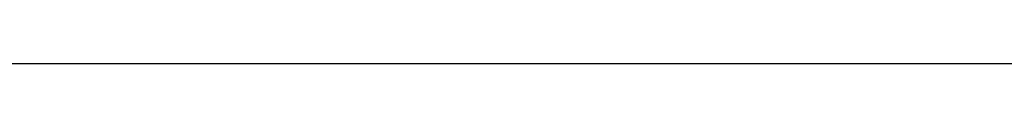
# Model space of a CAD drawing. Units: inches. Extents: x 2091 to 2899, y 967 to 2217.
# Tile 159 of 256: x 2192.883 to 2202.513, y 1152.247 to 1152.247. Entities that reach past the tile are written whole.
import ezdxf

# ---------------------------------------------------------------- set-up
doc = ezdxf.new("R2010")
doc.units = ezdxf.units.IN
doc.layers.add('A-ANNO-DIMS', color=2, linetype='Continuous', lineweight=18)
doc.styles.get("Standard").update_dxf_attribs({"font": 'arial.ttf'})
doc.dimstyles.new('ISO-25', dxfattribs={"dimtxt": 4, "dimasz": 4, "dimexe": 1.25, "dimexo": 0.625, "dimtad": 1, "dimdec": 0, "dimlunit": 3, "dimtxsty": 'Standard', "dimcen": 2.5, "dimadec": 0, "dimazin": 0, "dimtfac": 1, "dimtdec": 0, "dimtmove": 0, "dimatfit": 3, "dimfxl": 1, "dimarcsym": 0})

# ---------------------------------------------------------------- blocks, each defined once
blk = doc.blocks.new('*D91')
at = {"layer": 'A-ANNO-DIMS', "color": 0, "lineweight": -2, "transparency": 16777216}
for p, q in [((2211.6506, 1152.2471), (2098.3113, 1152.2471)), ((2099.5613, 1103.9191), (2099.5613, 1148.2471)), ((2211.5186, 1099.9191), (2098.3113, 1099.9191))]:
    blk.add_line(p, q, dxfattribs=at)
at = {"layer": 'A-ANNO-DIMS', "color": 0, "transparency": 16777216}
for points in [[(2098.8947, 1148.2471), (2100.228, 1148.2471), (2099.5613, 1152.2471)], [(2098.8947, 1103.9191), (2100.228, 1103.9191), (2099.5613, 1099.9191)]]:
    blk.add_solid(points, dxfattribs=at)
at = {"layer": 'Defpoints', "color": 0, "transparency": 16777216}
for p in [(2099.5613, 1152.2471), (2212.2756, 1152.2471), (2212.1436, 1099.9191)]:
    blk.add_point(p, dxfattribs=at)
at = {"layer": 'A-ANNO-DIMS', "color": 0, "transparency": 16777216, "insert": (2096.8681, 1126.0831), "char_height": 4, "attachment_point": 5, "rotation": 90}
blk.add_mtext('4\'-4 1/2"', dxfattribs=at)

msp = doc.modelspace()

# ---------------------------------------------------------------- dimensions: what is measured, and where the dimension line sits
at = {"layer": 'A-ANNO-DIMS'}
dim = msp.add_linear_dim(base=(2099.5613, 1152.2471), p1=(2212.1436, 1099.9191), p2=(2212.2756, 1152.2471), angle=90, dimstyle='ISO-25', override={"dimdec": 1, "dimlfac": 1, "dimrnd": 0, "dimzin": 1, "dimdsep": 46, "dimlunit": 4, "dimfrac": 2}, dxfattribs=at)
dim.commit()
dim.dimension.update_dxf_attribs({"geometry": '*D91', "text_midpoint": (2096.8681, 1126.0831)})

doc.saveas('drawing.dxf')
